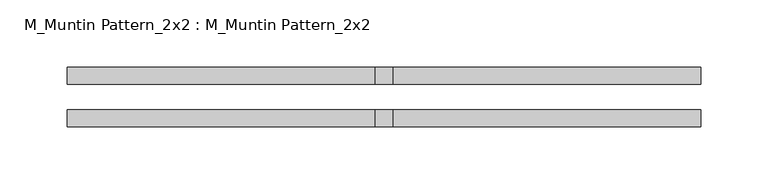
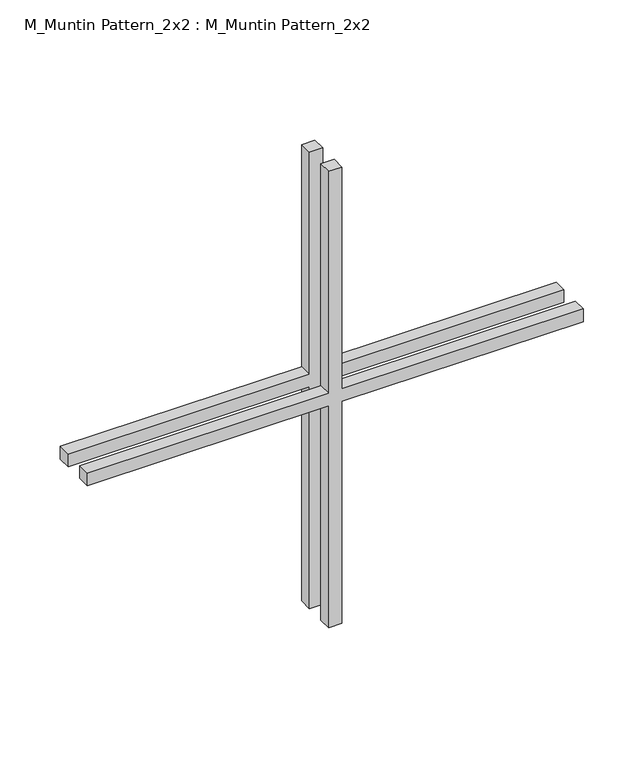
"""IFC4 building model written with IfcOpenShell, lengths in millimetres: proxy geometry, M_Muntin Pattern_2x2 : M_Muntin Pattern_2x2."""

from ifc_helpers import new_model, si_unit, frame, origin, place, context, project, spatial, polyline, outline, extrude, source, transform, mapped, element, save


def m_muntin_pattern_2x2_m_muntin_pattern_2x2_ec2ff75e(model_context):
    return source(origin(), model_context, "Body", "SweptSolid", [
        extrude(outline(polyline([(236.5, -6.35), (236.5, -236.5375), (223.8, -236.5375), (223.8, -6.35), (0.0, -6.35), (0.0, 6.35), (223.8, 6.35), (223.8, 236.5375), (236.5, 236.5375), (236.5, 6.35), (460.3, 6.35), (460.3, -6.35), (236.5, -6.35)])), frame((0.0, 9.525, 0.0), z_axis=(0.0, 1.0, 0.0), x_axis=(0.0, 0.0, 1.0)), (0.0, 0.0, 1.0), 12.7),
        extrude(outline(polyline([(236.5, -6.35), (236.5, -236.5375), (223.8, -236.5375), (223.8, -6.35), (0.0, -6.35), (0.0, 6.35), (223.8, 6.35), (223.8, 236.5375), (236.5, 236.5375), (236.5, 6.35), (460.3, 6.35), (460.3, -6.35), (236.5, -6.35)])), frame((0.0, -22.225, 0.0), z_axis=(0.0, 1.0, 0.0), x_axis=(0.0, 0.0, 1.0)), (0.0, 0.0, 1.0), 12.7),
    ])


if __name__ == "__main__":
    model = new_model("IFC4")
    model_context = context("Model", 3, world=origin())
    ifc_project = project(units=[si_unit("LENGTHUNIT", "METRE", prefix="MILLI")], contexts=[model_context])
    site = spatial("IfcSite", under=ifc_project)
    building = spatial("IfcBuilding", under=site)
    placement = place(None, origin())
    m_muntin_pattern_2x2_m_muntin_pattern_2x2_shape = m_muntin_pattern_2x2_m_muntin_pattern_2x2_ec2ff75e(model_context)
    element("IfcBuildingElementProxy", 1, Name="M_Muntin Pattern_2x2 : M_Muntin Pattern_2x2", ObjectType="M_Muntin Pattern_2x2 : M_Muntin Pattern_2x2", at=placement, inside=building, context=model_context, shape_type="MappedRepresentation", body=[
        mapped(m_muntin_pattern_2x2_m_muntin_pattern_2x2_shape, transform((0.0, 0.0, 0.0), x_axis=(1.0, 0.0, 0.0), y_axis=(0.0, 1.0, 0.0), z_axis=(0.0, 0.0, 1.0))),
    ])
    save(model, "model.ifc")

# Revit data of these elements
# Type "M_Muntin Pattern_2x2 : M_Muntin Pattern_2x2"
#   Width [instance default] = 3' - 11.24409"
#   Thickness = 0' - 0 1/2"
#   Height [instance default] = 3' - 11.24409"
#   Distance = 0' - 0 3/4"
#   Interior Material [instance default] = none
#   Exterior Material [instance default] = none
#   Default Elevation = 0
# Element 1 (IfcBuildingElementProxy, "M_Muntin Pattern_2x2 : M_Muntin Pattern_2x2")
#   Width = 1' - 6 5/8"
#   Height = 1' - 6.12205"
#   Interior Material = Wood - Stained
#   Exterior Material = Clad - White
#   Materials on its faces: "Clad - White", "Wood - Stained"
# Materials
#   "Clad - White": class "Wood", colour RGB 242 242 238, transparency 0, Cost = 0
#   "Wood - Stained": class "Wood", colour RGB 227 170 128, transparency 0, Cost = 0
